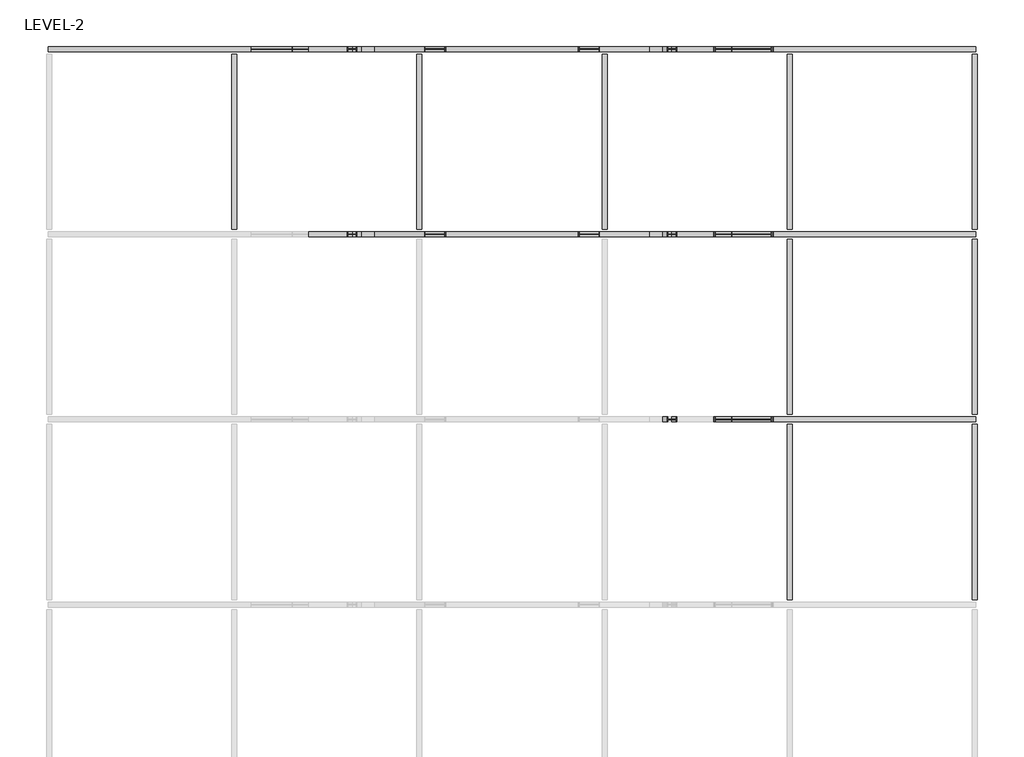
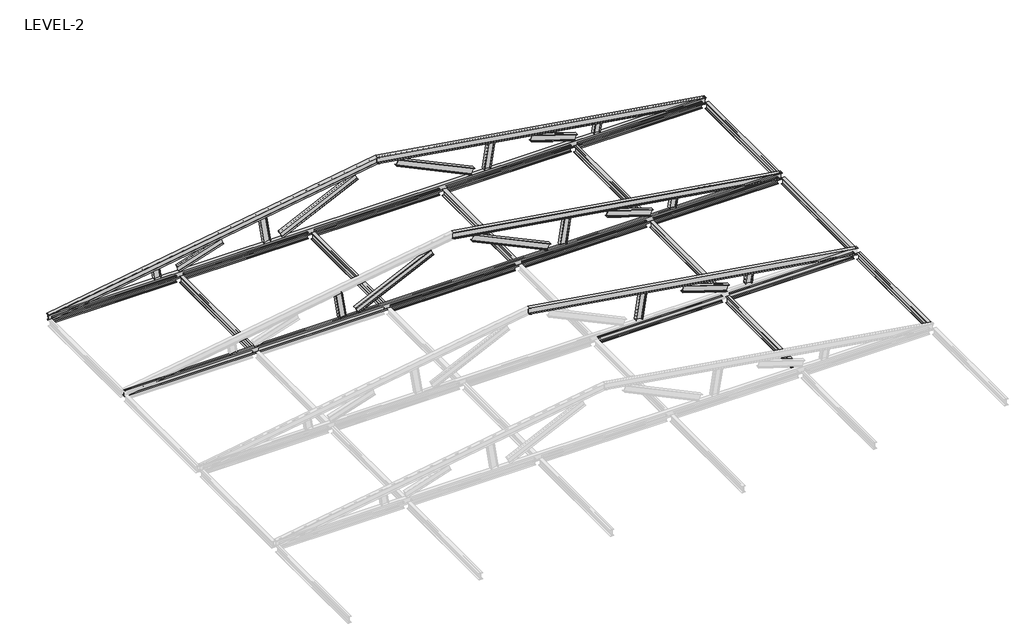
# One storey, part 3 of 3: 42 beams.
"""IFC4 building model written with IfcOpenShell, lengths in millimetres."""

from ifc_helpers import new_model, si_unit, frame, origin, place, context, project, spatial, polyline, circle_curve, ellipse_curve, transform, mapped, element, save
from ifc_brep_helpers import plane_surface, revolved_surface, advanced_brep
from components import ub_universal_beams_ub305x165x40_616d6e4e, ub_universal_beams_ub305x165x40_3f70edd5, ub_universal_beams_ub305x165x40_c9eec61f, ub_universal_beams_ub305x165x40_c956ba20, ub_universal_beams_ub305x165x40_f58164a9, ub_universal_beams_ub305x165x40_ef0a91e2, ub_universal_beams_ub305x165x40_83ed4f69, ub_universal_beams_ub305x165x40_46a3dc55, ub_universal_beams_ub305x165x40_0b6a72e4, ub_universal_beams_ub305x165x40_63d5ebb1, ub_universal_beams_ub305x165x40_05d28e63

model = new_model("IFC4")

# Units and contexts
model_context = context("Model", 3, world=origin())
ifc_project = project(units=[si_unit("LENGTHUNIT", "METRE", prefix="MILLI")], contexts=[model_context])

# Site, building, storey
site = spatial("IfcSite", under=ifc_project)
building = spatial("IfcBuilding", under=site)
storey = spatial("IfcBuildingStorey", under=building, Name="LEVEL-2", Elevation=4267.0)

# Beams
placement = place(None, origin())
element("IfcBeam", 1, ObjectType="UB-Universal Beams : UB305x165x40", at=placement, inside=storey, context=model_context, shape_type="AdvancedBrep", body=[
    advanced_brep(
    [(11917.6451312, 4042.0234105, 4127.2241081), (11917.6451312, 3971.4234105, 4127.2241081), (11919.0296431, 3962.5234105, 4136.0157591), (11960.2849884, 3962.5234105, 4397.9872012), (11961.6695003, 3971.4234105, 4406.7788522), (11961.6695003, 4042.0234105, 4406.7788522), (11963.2562444, 4042.0234105, 4416.8546768), (11963.2562444, 3877.0234105, 4416.8546768), (11961.6695003, 3877.0234105, 4406.7788522), (11961.6695003, 3947.6234105, 4406.7788522), (11960.2849884, 3956.5234105, 4397.9872012), (11919.0296431, 3956.5234105, 4136.0157591), (11917.6451312, 3947.6234105, 4127.2241081), (11917.6451312, 3877.0234105, 4127.2241081), (11916.0583871, 3877.0234105, 4117.1482834), (11916.0583871, 4042.0234105, 4117.1482834), (-3300.3332854, 4042.0234105, 6523.7561422), (-3300.3332854, 3971.4234105, 6523.7561422), (-3300.3332854, 3962.5234105, 6532.7658266), (-3300.3332854, 3962.5234105, 6801.2341734), (-3300.3332854, 3971.4234105, 6810.2438578), (-3300.3332854, 4042.0234105, 6810.2438578), (-3300.3332854, 4042.0234105, 6820.5695634), (-3300.3332854, 3877.0234105, 6820.5695634), (-3300.3332854, 3877.0234105, 6810.2438578), (-3300.3332854, 3947.6234105, 6810.2438578), (-3300.3332854, 3956.5234105, 6801.2341734), (-3300.3332854, 3956.5234105, 6532.7658266), (-3300.3332854, 3947.6234105, 6523.7561422), (-3300.3332854, 3877.0234105, 6523.7561422), (-3300.3332854, 3877.0234105, 6513.4304366), (-3300.3332854, 4042.0234105, 6513.4304366)],
    [
        (0, 1),
        (1, 2, circle_curve(frame((11919.0296431, 3971.4234105, 4136.0157591), z_axis=(-0.9878259507117182, 0.0, 0.1555631418443652), x_axis=(0.0, -1.0, 0.0)), 8.9)),
        (2, 3),
        (3, 4, circle_curve(frame((11960.2849884, 3971.4234105, 4397.9872012), z_axis=(-0.9878259507117182, 0.0, 0.1555631418443652), x_axis=(0.0, -1.0, 0.0)), 8.9)),
        (4, 5),
        (5, 6),
        (6, 7),
        (7, 8),
        (8, 9),
        (9, 10, circle_curve(frame((11960.2849884, 3947.6234105, 4397.9872012), z_axis=(-0.9878259507117182, 0.0, 0.1555631418443652), x_axis=(0.0, -1.0, 0.0)), 8.9)),
        (10, 11),
        (11, 12, circle_curve(frame((11919.0296431, 3947.6234105, 4136.0157591), z_axis=(-0.9878259507117182, 0.0, 0.1555631418443652), x_axis=(0.0, -1.0, 0.0)), 8.9)),
        (12, 13),
        (13, 14),
        (14, 15),
        (15, 0),
        (0, 16),
        (16, 17),
        (17, 1),
        (17, 18, ellipse_curve(frame((-3300.3332854, 3971.4234105, 6532.7658266), z_axis=(-1.0, 0.0, 0.0), x_axis=(0.0, 0.0, 1.0)), 9.0096843, 8.9)),
        (18, 2),
        (18, 19),
        (19, 3),
        (19, 20, ellipse_curve(frame((-3300.3332854, 3971.4234105, 6801.2341734), z_axis=(-1.0, 0.0, 0.0), x_axis=(0.0, 0.0, 1.0)), 9.0096843, 8.9)),
        (20, 4),
        (20, 21),
        (21, 5),
        (21, 22),
        (22, 6),
        (22, 23),
        (23, 7),
        (23, 24),
        (24, 8),
        (24, 25),
        (25, 9),
        (25, 26, ellipse_curve(frame((-3300.3332854, 3947.6234105, 6801.2341734), z_axis=(-1.0, 0.0, 0.0), x_axis=(0.0, 0.0, 1.0)), 9.0096843, 8.9)),
        (26, 10),
        (26, 27),
        (27, 11),
        (27, 28, ellipse_curve(frame((-3300.3332854, 3947.6234105, 6532.7658266), z_axis=(-1.0, 0.0, 0.0), x_axis=(0.0, 0.0, 1.0)), 9.0096843, 8.9)),
        (28, 12),
        (28, 29),
        (29, 13),
        (29, 30),
        (30, 14),
        (30, 31),
        (31, 15),
        (31, 16),
    ],
    [
        plane_surface(frame((11939.6573157, 3959.5234105, 4267.0014801), z_axis=(0.9878259507117182, 0.0, -0.1555631418443652), x_axis=(0.1555631418443652, 0.0, 0.9878259507117182))),
        plane_surface(frame((11917.6451312, 4042.0234105, 4127.2241081), z_axis=(0.1555631418443652, 0.0, 0.9878259507117182), x_axis=(-0.9878259507117182, 0.0, 0.1555631418443652))),
        revolved_surface(polyline([(-3301.7177973591024, 3962.5234105, 6532.983859959702), (11919.029643166847, 3962.5234105, 4136.015759089472)]), (11919.0296431, 3971.4234105, 4136.0157591), (-0.9878259507117182, 0.0, 0.1555631418443652)),
        plane_surface(frame((11919.0296431, 3962.5234105, 4136.0157591), z_axis=(0.0, 1.0, 0.0), x_axis=(-0.9878259507117182, 0.0, 0.1555631418443652))),
        revolved_surface(polyline([(-3301.717797363457, 3962.5234105, 6801.452206832042), (11960.2849884, 3962.5234105, 4397.9872012)]), (11960.2849884, 3971.4234105, 4397.9872012), (-0.9878259507117182, 0.0, 0.1555631418443652)),
        plane_surface(frame((11961.6695003, 3971.4234105, 4406.7788522), z_axis=(-0.1555631418443652, 0.0, -0.9878259507117182), x_axis=(-0.9878259507117182, 0.0, 0.1555631418443652))),
        plane_surface(frame((11961.6695003, 4042.0234105, 4406.7788522), z_axis=(0.0, 1.0, 0.0), x_axis=(-0.9878259507117182, 0.0, 0.1555631418443652))),
        plane_surface(frame((11963.2562444, 4042.0234105, 4416.8546768), z_axis=(0.1555631418443652, 0.0, 0.9878259507117182), x_axis=(-0.9878259507117182, 0.0, 0.1555631418443652))),
        plane_surface(frame((11963.2562444, 3877.0234105, 4416.8546768), z_axis=(0.0, -1.0, 0.0), x_axis=(-0.9878259507117182, 0.0, 0.1555631418443652))),
        plane_surface(frame((11961.6695003, 3877.0234105, 4406.7788522), z_axis=(-0.1555631418443652, 0.0, -0.9878259507117182), x_axis=(-0.9878259507117182, 0.0, 0.1555631418443652))),
        revolved_surface(polyline([(-3301.717797363457, 3938.7234104999998, 6801.452206832042), (11960.2849884, 3938.7234104999998, 4397.9872012)]), (11960.2849884, 3947.6234105, 4397.9872012), (-0.9878259507117182, 0.0, 0.1555631418443652)),
        plane_surface(frame((11960.2849884, 3956.5234105, 4397.9872012), z_axis=(0.0, -1.0, 0.0), x_axis=(-0.9878259507117182, 0.0, 0.1555631418443652))),
        revolved_surface(polyline([(-3301.7177973591024, 3938.7234104999998, 6532.983859959702), (11919.029643166847, 3938.7234104999998, 4136.015759089472)]), (11919.0296431, 3947.6234105, 4136.0157591), (-0.9878259507117182, 0.0, 0.1555631418443652)),
        plane_surface(frame((11917.6451312, 3947.6234105, 4127.2241081), z_axis=(0.1555631418443652, 0.0, 0.9878259507117182), x_axis=(-0.9878259507117182, 0.0, 0.1555631418443652))),
        plane_surface(frame((11917.6451312, 3877.0234105, 4127.2241081), z_axis=(0.0, -1.0, 0.0), x_axis=(-0.9878259507117182, 0.0, 0.1555631418443652))),
        plane_surface(frame((11916.0583871, 3877.0234105, 4117.1482834), z_axis=(-0.1555631418443652, 0.0, -0.9878259507117182), x_axis=(-0.9878259507117182, 0.0, 0.1555631418443652))),
        plane_surface(frame((11916.0583871, 4042.0234105, 4117.1482834), z_axis=(0.0, 1.0, 0.0), x_axis=(-0.9878259507117182, 0.0, 0.1555631418443652))),
        plane_surface(frame((-3300.3332854, 3959.5234105, 6820.5695634), z_axis=(-1.0, 0.0, 0.0), x_axis=(0.0, 1.0, 0.0))),
    ],
    [
        (0, [[1, 2, 3, 4, 5, 6, 7, 8, 9, 10, 11, 12, 13, 14, 15, 16]]),
        (1, [[-1, 17, 18, 19]]),
        (2, [[-2, -19, 20, 21]]),
        (3, [[-3, -21, 22, 23]]),
        (4, [[-4, -23, 24, 25]]),
        (5, [[-5, -25, 26, 27]]),
        (6, [[-6, -27, 28, 29]]),
        (7, [[-7, -29, 30, 31]]),
        (8, [[-8, -31, 32, 33]]),
        (9, [[-9, -33, 34, 35]]),
        (10, [[-10, -35, 36, 37]]),
        (11, [[-11, -37, 38, 39]]),
        (12, [[-12, -39, 40, 41]]),
        (13, [[-13, -41, 42, 43]]),
        (14, [[-14, -43, 44, 45]]),
        (15, [[-15, -45, 46, 47]]),
        (16, [[-16, -47, 48, -17]]),
        (17, [[-48, -46, -44, -42, -40, -38, -36, -34, -32, -30, -28, -26, -24, -22, -20, -18]]),
    ],
),
])
element("IfcBeam", 2, ObjectType="UB-Universal Beams : UB305x165x40", at=placement, inside=storey, context=model_context, shape_type="AdvancedBrep", body=[
    advanced_brep(
    [(11917.6451312, 10138.0234105, 4127.2241081), (11917.6451312, 10067.4234105, 4127.2241081), (11919.0296431, 10058.5234105, 4136.0157591), (11960.2849884, 10058.5234105, 4397.9872012), (11961.6695003, 10067.4234105, 4406.7788522), (11961.6695003, 10138.0234105, 4406.7788522), (11963.2562444, 10138.0234105, 4416.8546768), (11963.2562444, 9973.0234105, 4416.8546768), (11961.6695003, 9973.0234105, 4406.7788522), (11961.6695003, 10043.6234105, 4406.7788522), (11960.2849884, 10052.5234105, 4397.9872012), (11919.0296431, 10052.5234105, 4136.0157591), (11917.6451312, 10043.6234105, 4127.2241081), (11917.6451312, 9973.0234105, 4127.2241081), (11916.0583871, 9973.0234105, 4117.1482834), (11916.0583871, 10138.0234105, 4117.1482834), (-3300.3332854, 10138.0234105, 6523.7561422), (-3300.3332854, 10067.4234105, 6523.7561422), (-3300.3332854, 10058.5234105, 6532.7658266), (-3300.3332854, 10058.5234105, 6801.2341734), (-3300.3332854, 10067.4234105, 6810.2438578), (-3300.3332854, 10138.0234105, 6810.2438578), (-3300.3332854, 10138.0234105, 6820.5695634), (-3300.3332854, 9973.0234105, 6820.5695634), (-3300.3332854, 9973.0234105, 6810.2438578), (-3300.3332854, 10043.6234105, 6810.2438578), (-3300.3332854, 10052.5234105, 6801.2341734), (-3300.3332854, 10052.5234105, 6532.7658266), (-3300.3332854, 10043.6234105, 6523.7561422), (-3300.3332854, 9973.0234105, 6523.7561422), (-3300.3332854, 9973.0234105, 6513.4304366), (-3300.3332854, 10138.0234105, 6513.4304366)],
    [
        (0, 1),
        (1, 2, circle_curve(frame((11919.0296431, 10067.4234105, 4136.0157591), z_axis=(-0.9878259507117182, 0.0, 0.1555631418443652), x_axis=(0.0, -1.0, 0.0)), 8.9)),
        (2, 3),
        (3, 4, circle_curve(frame((11960.2849884, 10067.4234105, 4397.9872012), z_axis=(-0.9878259507117182, 0.0, 0.1555631418443652), x_axis=(0.0, -1.0, 0.0)), 8.9)),
        (4, 5),
        (5, 6),
        (6, 7),
        (7, 8),
        (8, 9),
        (9, 10, circle_curve(frame((11960.2849884, 10043.6234105, 4397.9872012), z_axis=(-0.9878259507117182, 0.0, 0.1555631418443652), x_axis=(0.0, -1.0, 0.0)), 8.9)),
        (10, 11),
        (11, 12, circle_curve(frame((11919.0296431, 10043.6234105, 4136.0157591), z_axis=(-0.9878259507117182, 0.0, 0.1555631418443652), x_axis=(0.0, -1.0, 0.0)), 8.9)),
        (12, 13),
        (13, 14),
        (14, 15),
        (15, 0),
        (0, 16),
        (16, 17),
        (17, 1),
        (17, 18, ellipse_curve(frame((-3300.3332854, 10067.4234105, 6532.7658266), z_axis=(-1.0, 0.0, 0.0), x_axis=(0.0, 0.0, 1.0)), 9.0096843, 8.9)),
        (18, 2),
        (18, 19),
        (19, 3),
        (19, 20, ellipse_curve(frame((-3300.3332854, 10067.4234105, 6801.2341734), z_axis=(-1.0, 0.0, 0.0), x_axis=(0.0, 0.0, 1.0)), 9.0096843, 8.9)),
        (20, 4),
        (20, 21),
        (21, 5),
        (21, 22),
        (22, 6),
        (22, 23),
        (23, 7),
        (23, 24),
        (24, 8),
        (24, 25),
        (25, 9),
        (25, 26, ellipse_curve(frame((-3300.3332854, 10043.6234105, 6801.2341734), z_axis=(-1.0, 0.0, 0.0), x_axis=(0.0, 0.0, 1.0)), 9.0096843, 8.9)),
        (26, 10),
        (26, 27),
        (27, 11),
        (27, 28, ellipse_curve(frame((-3300.3332854, 10043.6234105, 6532.7658266), z_axis=(-1.0, 0.0, 0.0), x_axis=(0.0, 0.0, 1.0)), 9.0096843, 8.9)),
        (28, 12),
        (28, 29),
        (29, 13),
        (29, 30),
        (30, 14),
        (30, 31),
        (31, 15),
        (31, 16),
    ],
    [
        plane_surface(frame((11939.6573157, 10055.5234105, 4267.0014801), z_axis=(0.9878259507117182, 0.0, -0.1555631418443652), x_axis=(0.1555631418443652, 0.0, 0.9878259507117182))),
        plane_surface(frame((11917.6451312, 10138.0234105, 4127.2241081), z_axis=(0.1555631418443652, 0.0, 0.9878259507117182), x_axis=(-0.9878259507117182, 0.0, 0.1555631418443652))),
        revolved_surface(polyline([(-3301.7177973591024, 10058.5234105, 6532.983859959702), (11919.029643166847, 10058.5234105, 4136.015759089472)]), (11919.0296431, 10067.4234105, 4136.0157591), (-0.9878259507117182, 0.0, 0.1555631418443652)),
        plane_surface(frame((11919.0296431, 10058.5234105, 4136.0157591), z_axis=(0.0, 1.0, 0.0), x_axis=(-0.9878259507117182, 0.0, 0.1555631418443652))),
        revolved_surface(polyline([(-3301.717797363457, 10058.5234105, 6801.452206832042), (11960.2849884, 10058.5234105, 4397.9872012)]), (11960.2849884, 10067.4234105, 4397.9872012), (-0.9878259507117182, 0.0, 0.1555631418443652)),
        plane_surface(frame((11961.6695003, 10067.4234105, 4406.7788522), z_axis=(-0.1555631418443652, 0.0, -0.9878259507117182), x_axis=(-0.9878259507117182, 0.0, 0.1555631418443652))),
        plane_surface(frame((11961.6695003, 10138.0234105, 4406.7788522), z_axis=(0.0, 1.0, 0.0), x_axis=(-0.9878259507117182, 0.0, 0.1555631418443652))),
        plane_surface(frame((11963.2562444, 10138.0234105, 4416.8546768), z_axis=(0.1555631418443652, 0.0, 0.9878259507117182), x_axis=(-0.9878259507117182, 0.0, 0.1555631418443652))),
        plane_surface(frame((11963.2562444, 9973.0234105, 4416.8546768), z_axis=(0.0, -1.0, 0.0), x_axis=(-0.9878259507117182, 0.0, 0.1555631418443652))),
        plane_surface(frame((11961.6695003, 9973.0234105, 4406.7788522), z_axis=(-0.1555631418443652, 0.0, -0.9878259507117182), x_axis=(-0.9878259507117182, 0.0, 0.1555631418443652))),
        revolved_surface(polyline([(-3301.717797363457, 10034.7234105, 6801.452206832042), (11960.2849884, 10034.7234105, 4397.9872012)]), (11960.2849884, 10043.6234105, 4397.9872012), (-0.9878259507117182, 0.0, 0.1555631418443652)),
        plane_surface(frame((11960.2849884, 10052.5234105, 4397.9872012), z_axis=(0.0, -1.0, 0.0), x_axis=(-0.9878259507117182, 0.0, 0.1555631418443652))),
        revolved_surface(polyline([(-3301.7177973591024, 10034.7234105, 6532.983859959702), (11919.029643166847, 10034.7234105, 4136.015759089472)]), (11919.0296431, 10043.6234105, 4136.0157591), (-0.9878259507117182, 0.0, 0.1555631418443652)),
        plane_surface(frame((11917.6451312, 10043.6234105, 4127.2241081), z_axis=(0.1555631418443652, 0.0, 0.9878259507117182), x_axis=(-0.9878259507117182, 0.0, 0.1555631418443652))),
        plane_surface(frame((11917.6451312, 9973.0234105, 4127.2241081), z_axis=(0.0, -1.0, 0.0), x_axis=(-0.9878259507117182, 0.0, 0.1555631418443652))),
        plane_surface(frame((11916.0583871, 9973.0234105, 4117.1482834), z_axis=(-0.1555631418443652, 0.0, -0.9878259507117182), x_axis=(-0.9878259507117182, 0.0, 0.1555631418443652))),
        plane_surface(frame((11916.0583871, 10138.0234105, 4117.1482834), z_axis=(0.0, 1.0, 0.0), x_axis=(-0.9878259507117182, 0.0, 0.1555631418443652))),
        plane_surface(frame((-3300.3332854, 10055.5234105, 6820.5695634), z_axis=(-1.0, 0.0, 0.0), x_axis=(0.0, 1.0, 0.0))),
    ],
    [
        (0, [[1, 2, 3, 4, 5, 6, 7, 8, 9, 10, 11, 12, 13, 14, 15, 16]]),
        (1, [[-1, 17, 18, 19]]),
        (2, [[-2, -19, 20, 21]]),
        (3, [[-3, -21, 22, 23]]),
        (4, [[-4, -23, 24, 25]]),
        (5, [[-5, -25, 26, 27]]),
        (6, [[-6, -27, 28, 29]]),
        (7, [[-7, -29, 30, 31]]),
        (8, [[-8, -31, 32, 33]]),
        (9, [[-9, -33, 34, 35]]),
        (10, [[-10, -35, 36, 37]]),
        (11, [[-11, -37, 38, 39]]),
        (12, [[-12, -39, 40, 41]]),
        (13, [[-13, -41, 42, 43]]),
        (14, [[-14, -43, 44, 45]]),
        (15, [[-15, -45, 46, 47]]),
        (16, [[-16, -47, 48, -17]]),
        (17, [[-48, -46, -44, -42, -40, -38, -36, -34, -32, -30, -28, -26, -24, -22, -20, -18]]),
    ],
),
])
element("IfcBeam", 3, ObjectType="UB-Universal Beams : UB305x165x40", at=placement, inside=storey, context=model_context, shape_type="AdvancedBrep", body=[
    advanced_brep(
    [(-18518.3117021, 16234.0234105, 4127.2241081), (-18516.724958, 16234.0234105, 4117.1482834), (-18516.724958, 16069.0234105, 4117.1482834), (-18518.3117021, 16069.0234105, 4127.2241081), (-18518.3117021, 16139.6234105, 4127.2241081), (-18519.696214, 16148.5234105, 4136.0157591), (-18560.9515593, 16148.5234105, 4397.9872012), (-18562.3360712, 16139.6234105, 4406.7788522), (-18562.3360712, 16069.0234105, 4406.7788522), (-18563.9228153, 16069.0234105, 4416.8546768), (-18563.9228153, 16234.0234105, 4416.8546768), (-18562.3360712, 16234.0234105, 4406.7788522), (-18562.3360712, 16163.4234105, 4406.7788522), (-18560.9515593, 16154.5234105, 4397.9872012), (-18519.696214, 16154.5234105, 4136.0157591), (-18518.3117021, 16163.4234105, 4127.2241081), (-3300.3332854, 16163.4234105, 6523.7561422), (-3300.3332854, 16234.0234105, 6523.7561422), (-3300.3332854, 16154.5234105, 6532.7658266), (-3300.3332854, 16154.5234105, 6801.2341734), (-3300.3332854, 16163.4234105, 6810.2438578), (-3300.3332854, 16234.0234105, 6810.2438578), (-3300.3332854, 16234.0234105, 6820.5695634), (-3300.3332854, 16069.0234105, 6820.5695634), (-3300.3332854, 16069.0234105, 6810.2438578), (-3300.3332854, 16139.6234105, 6810.2438578), (-3300.3332854, 16148.5234105, 6801.2341734), (-3300.3332854, 16148.5234105, 6532.7658266), (-3300.3332854, 16139.6234105, 6523.7561422), (-3300.3332854, 16069.0234105, 6523.7561422), (-3300.3332854, 16069.0234105, 6513.4304366), (-3300.3332854, 16234.0234105, 6513.4304366)],
    [
        (0, 1),
        (1, 2),
        (2, 3),
        (3, 4),
        (4, 5, circle_curve(frame((-18519.696214, 16139.6234105, 4136.0157591), z_axis=(0.9878259507117182, 0.0, 0.1555631418443652), x_axis=(0.0, -1.0, 0.0)), 8.9)),
        (5, 6),
        (6, 7, circle_curve(frame((-18560.9515593, 16139.6234105, 4397.9872012), z_axis=(0.9878259507117182, 0.0, 0.1555631418443652), x_axis=(0.0, -1.0, 0.0)), 8.9)),
        (7, 8),
        (8, 9),
        (9, 10),
        (10, 11),
        (11, 12),
        (12, 13, circle_curve(frame((-18560.9515593, 16163.4234105, 4397.9872012), z_axis=(0.9878259507117182, 0.0, 0.1555631418443652), x_axis=(0.0, -1.0, 0.0)), 8.9)),
        (13, 14),
        (14, 15, circle_curve(frame((-18519.696214, 16163.4234105, 4136.0157591), z_axis=(0.9878259507117182, 0.0, 0.1555631418443652), x_axis=(0.0, -1.0, 0.0)), 8.9)),
        (15, 0),
        (16, 17),
        (17, 0),
        (15, 16),
        (18, 16, ellipse_curve(frame((-3300.3332854, 16163.4234105, 6532.7658266), z_axis=(1.0, 0.0, 0.0), x_axis=(0.0, 0.0, -1.0)), 9.0096843, 8.9)),
        (14, 18),
        (19, 18),
        (13, 19),
        (20, 19, ellipse_curve(frame((-3300.3332854, 16163.4234105, 6801.2341734), z_axis=(1.0, 0.0, 0.0), x_axis=(0.0, 0.0, -1.0)), 9.0096843, 8.9)),
        (12, 20),
        (21, 20),
        (11, 21),
        (22, 21),
        (10, 22),
        (23, 22),
        (9, 23),
        (24, 23),
        (8, 24),
        (25, 24),
        (7, 25),
        (26, 25, ellipse_curve(frame((-3300.3332854, 16139.6234105, 6801.2341734), z_axis=(1.0, 0.0, 0.0), x_axis=(0.0, 0.0, -1.0)), 9.0096843, 8.9)),
        (6, 26),
        (27, 26),
        (5, 27),
        (28, 27, ellipse_curve(frame((-3300.3332854, 16139.6234105, 6532.7658266), z_axis=(1.0, 0.0, 0.0), x_axis=(0.0, 0.0, -1.0)), 9.0096843, 8.9)),
        (4, 28),
        (29, 28),
        (3, 29),
        (30, 29),
        (2, 30),
        (31, 30),
        (1, 31),
        (17, 31),
    ],
    [
        plane_surface(frame((-18540.3238866, 16151.5234105, 4267.0014801), z_axis=(-0.9878259507117182, 0.0, -0.1555631418443652), x_axis=(-0.1555631418443652, 0.0, 0.9878259507117182))),
        plane_surface(frame((-3278.3304997, 16234.0234105, 6527.2211478), z_axis=(-0.1555631418443652, 0.0, 0.9878259507117182), x_axis=(-0.9878259507117182, 0.0, -0.1555631418443652))),
        revolved_surface(polyline([(-18519.696214059466, 16154.5234105, 4136.015759042602), (-3298.948773435937, 16154.5234105, 6532.983859928199)]), (-3279.7150116, 16163.4234105, 6536.0127988), (-0.9878259507117182, 0.0, -0.1555631418443652)),
        plane_surface(frame((-3279.7150116, 16154.5234105, 6536.0127988), z_axis=(0.0, 1.0, 0.0), x_axis=(-0.9878259507117182, 0.0, -0.1555631418443652))),
        revolved_surface(polyline([(-18560.95155929262, 16154.5234105, 4397.98720115313), (-3298.948773431581, 16154.5234105, 6801.452206800539)]), (-3320.9703569, 16163.4234105, 6797.9842409), (-0.9878259507117182, 0.0, -0.1555631418443652)),
        plane_surface(frame((-3322.3548688, 16163.4234105, 6806.7758919), z_axis=(0.1555631418443652, 0.0, -0.9878259507117182), x_axis=(-0.9878259507117182, 0.0, -0.1555631418443652))),
        plane_surface(frame((-3322.3548688, 16234.0234105, 6806.7758919), z_axis=(0.0, 1.0, 0.0), x_axis=(-0.9878259507117182, 0.0, -0.1555631418443652))),
        plane_surface(frame((-3323.9416129, 16234.0234105, 6816.8517166), z_axis=(-0.1555631418443652, 0.0, 0.9878259507117182), x_axis=(-0.9878259507117182, 0.0, -0.1555631418443652))),
        plane_surface(frame((-3323.9416129, 16069.0234105, 6816.8517166), z_axis=(0.0, -1.0, 0.0), x_axis=(-0.9878259507117182, 0.0, -0.1555631418443652))),
        plane_surface(frame((-3322.3548688, 16069.0234105, 6806.7758919), z_axis=(0.1555631418443652, 0.0, -0.9878259507117182), x_axis=(-0.9878259507117182, 0.0, -0.1555631418443652))),
        revolved_surface(polyline([(-18560.95155929262, 16130.7234105, 4397.98720115313), (-3298.948773431581, 16130.7234105, 6801.452206800539)]), (-3320.9703569, 16139.6234105, 6797.9842409), (-0.9878259507117182, 0.0, -0.1555631418443652)),
        plane_surface(frame((-3320.9703569, 16148.5234105, 6797.9842409), z_axis=(0.0, -1.0, 0.0), x_axis=(-0.9878259507117182, 0.0, -0.1555631418443652))),
        revolved_surface(polyline([(-18519.696214059466, 16130.7234105, 4136.015759042602), (-3298.948773435937, 16130.7234105, 6532.983859928199)]), (-3279.7150116, 16139.6234105, 6536.0127988), (-0.9878259507117182, 0.0, -0.1555631418443652)),
        plane_surface(frame((-3278.3304997, 16139.6234105, 6527.2211478), z_axis=(-0.1555631418443652, 0.0, 0.9878259507117182), x_axis=(-0.9878259507117182, 0.0, -0.1555631418443652))),
        plane_surface(frame((-3278.3304997, 16069.0234105, 6527.2211478), z_axis=(0.0, -1.0, 0.0), x_axis=(-0.9878259507117182, 0.0, -0.1555631418443652))),
        plane_surface(frame((-3276.7437556, 16069.0234105, 6517.1453232), z_axis=(0.1555631418443652, 0.0, -0.9878259507117182), x_axis=(-0.9878259507117182, 0.0, -0.1555631418443652))),
        plane_surface(frame((-3276.7437556, 16234.0234105, 6517.1453232), z_axis=(0.0, 1.0, 0.0), x_axis=(-0.9878259507117182, 0.0, -0.1555631418443652))),
        plane_surface(frame((-3300.3332854, 16151.5234105, 6820.5695634), z_axis=(1.0, 0.0, 0.0), x_axis=(0.0, -1.0, 0.0))),
    ],
    [
        (0, [[1, 2, 3, 4, 5, 6, 7, 8, 9, 10, 11, 12, 13, 14, 15, 16]]),
        (1, [[17, 18, -16, 19]]),
        (2, [[20, -19, -15, 21]]),
        (3, [[22, -21, -14, 23]]),
        (4, [[24, -23, -13, 25]]),
        (5, [[26, -25, -12, 27]]),
        (6, [[28, -27, -11, 29]]),
        (7, [[30, -29, -10, 31]]),
        (8, [[32, -31, -9, 33]]),
        (9, [[34, -33, -8, 35]]),
        (10, [[36, -35, -7, 37]]),
        (11, [[38, -37, -6, 39]]),
        (12, [[40, -39, -5, 41]]),
        (13, [[42, -41, -4, 43]]),
        (14, [[44, -43, -3, 45]]),
        (15, [[46, -45, -2, 47]]),
        (16, [[48, -47, -1, -18]]),
        (17, [[-17, -20, -22, -24, -26, -28, -30, -32, -34, -36, -38, -40, -42, -44, -46, -48]]),
    ],
),
])
element("IfcBeam", 4, ObjectType="UB-Universal Beams : UB305x165x40", at=placement, inside=storey, context=model_context, shape_type="AdvancedBrep", body=[
    advanced_brep(
    [(11917.6451312, 16234.0234105, 4127.2241081), (11917.6451312, 16163.4234105, 4127.2241081), (11919.0296431, 16154.5234105, 4136.0157591), (11960.2849884, 16154.5234105, 4397.9872012), (11961.6695003, 16163.4234105, 4406.7788522), (11961.6695003, 16234.0234105, 4406.7788522), (11963.2562444, 16234.0234105, 4416.8546768), (11963.2562444, 16069.0234105, 4416.8546768), (11961.6695003, 16069.0234105, 4406.7788522), (11961.6695003, 16139.6234105, 4406.7788522), (11960.2849884, 16148.5234105, 4397.9872012), (11919.0296431, 16148.5234105, 4136.0157591), (11917.6451312, 16139.6234105, 4127.2241081), (11917.6451312, 16069.0234105, 4127.2241081), (11916.0583871, 16069.0234105, 4117.1482834), (11916.0583871, 16234.0234105, 4117.1482834), (-3300.3332854, 16234.0234105, 6523.7561422), (-3300.3332854, 16163.4234105, 6523.7561422), (-3300.3332854, 16154.5234105, 6532.7658266), (-3300.3332854, 16154.5234105, 6801.2341734), (-3300.3332854, 16163.4234105, 6810.2438578), (-3300.3332854, 16234.0234105, 6810.2438578), (-3300.3332854, 16234.0234105, 6820.5695634), (-3300.3332854, 16069.0234105, 6820.5695634), (-3300.3332854, 16069.0234105, 6810.2438578), (-3300.3332854, 16139.6234105, 6810.2438578), (-3300.3332854, 16148.5234105, 6801.2341734), (-3300.3332854, 16148.5234105, 6532.7658266), (-3300.3332854, 16139.6234105, 6523.7561422), (-3300.3332854, 16069.0234105, 6523.7561422), (-3300.3332854, 16069.0234105, 6513.4304366), (-3300.3332854, 16234.0234105, 6513.4304366)],
    [
        (0, 1),
        (1, 2, circle_curve(frame((11919.0296431, 16163.4234105, 4136.0157591), z_axis=(-0.9878259507117182, 0.0, 0.1555631418443652), x_axis=(0.0, -1.0, 0.0)), 8.9)),
        (2, 3),
        (3, 4, circle_curve(frame((11960.2849884, 16163.4234105, 4397.9872012), z_axis=(-0.9878259507117182, 0.0, 0.1555631418443652), x_axis=(0.0, -1.0, 0.0)), 8.9)),
        (4, 5),
        (5, 6),
        (6, 7),
        (7, 8),
        (8, 9),
        (9, 10, circle_curve(frame((11960.2849884, 16139.6234105, 4397.9872012), z_axis=(-0.9878259507117182, 0.0, 0.1555631418443652), x_axis=(0.0, -1.0, 0.0)), 8.9)),
        (10, 11),
        (11, 12, circle_curve(frame((11919.0296431, 16139.6234105, 4136.0157591), z_axis=(-0.9878259507117182, 0.0, 0.1555631418443652), x_axis=(0.0, -1.0, 0.0)), 8.9)),
        (12, 13),
        (13, 14),
        (14, 15),
        (15, 0),
        (0, 16),
        (16, 17),
        (17, 1),
        (17, 18, ellipse_curve(frame((-3300.3332854, 16163.4234105, 6532.7658266), z_axis=(-1.0, 0.0, 0.0), x_axis=(0.0, 0.0, 1.0)), 9.0096843, 8.9)),
        (18, 2),
        (18, 19),
        (19, 3),
        (19, 20, ellipse_curve(frame((-3300.3332854, 16163.4234105, 6801.2341734), z_axis=(-1.0, 0.0, 0.0), x_axis=(0.0, 0.0, 1.0)), 9.0096843, 8.9)),
        (20, 4),
        (20, 21),
        (21, 5),
        (21, 22),
        (22, 6),
        (22, 23),
        (23, 7),
        (23, 24),
        (24, 8),
        (24, 25),
        (25, 9),
        (25, 26, ellipse_curve(frame((-3300.3332854, 16139.6234105, 6801.2341734), z_axis=(-1.0, 0.0, 0.0), x_axis=(0.0, 0.0, 1.0)), 9.0096843, 8.9)),
        (26, 10),
        (26, 27),
        (27, 11),
        (27, 28, ellipse_curve(frame((-3300.3332854, 16139.6234105, 6532.7658266), z_axis=(-1.0, 0.0, 0.0), x_axis=(0.0, 0.0, 1.0)), 9.0096843, 8.9)),
        (28, 12),
        (28, 29),
        (29, 13),
        (29, 30),
        (30, 14),
        (30, 31),
        (31, 15),
        (31, 16),
    ],
    [
        plane_surface(frame((11939.6573157, 16151.5234105, 4267.0014801), z_axis=(0.9878259507117182, 0.0, -0.1555631418443652), x_axis=(0.1555631418443652, 0.0, 0.9878259507117182))),
        plane_surface(frame((11917.6451312, 16234.0234105, 4127.2241081), z_axis=(0.1555631418443652, 0.0, 0.9878259507117182), x_axis=(-0.9878259507117182, 0.0, 0.1555631418443652))),
        revolved_surface(polyline([(-3301.7177973591024, 16154.5234105, 6532.983859959702), (11919.029643166847, 16154.5234105, 4136.015759089472)]), (11919.0296431, 16163.4234105, 4136.0157591), (-0.9878259507117182, 0.0, 0.1555631418443652)),
        plane_surface(frame((11919.0296431, 16154.5234105, 4136.0157591), z_axis=(0.0, 1.0, 0.0), x_axis=(-0.9878259507117182, 0.0, 0.1555631418443652))),
        revolved_surface(polyline([(-3301.717797363457, 16154.5234105, 6801.452206832042), (11960.2849884, 16154.5234105, 4397.9872012)]), (11960.2849884, 16163.4234105, 4397.9872012), (-0.9878259507117182, 0.0, 0.1555631418443652)),
        plane_surface(frame((11961.6695003, 16163.4234105, 4406.7788522), z_axis=(-0.1555631418443652, 0.0, -0.9878259507117182), x_axis=(-0.9878259507117182, 0.0, 0.1555631418443652))),
        plane_surface(frame((11961.6695003, 16234.0234105, 4406.7788522), z_axis=(0.0, 1.0, 0.0), x_axis=(-0.9878259507117182, 0.0, 0.1555631418443652))),
        plane_surface(frame((11963.2562444, 16234.0234105, 4416.8546768), z_axis=(0.1555631418443652, 0.0, 0.9878259507117182), x_axis=(-0.9878259507117182, 0.0, 0.1555631418443652))),
        plane_surface(frame((11963.2562444, 16069.0234105, 4416.8546768), z_axis=(0.0, -1.0, 0.0), x_axis=(-0.9878259507117182, 0.0, 0.1555631418443652))),
        plane_surface(frame((11961.6695003, 16069.0234105, 4406.7788522), z_axis=(-0.1555631418443652, 0.0, -0.9878259507117182), x_axis=(-0.9878259507117182, 0.0, 0.1555631418443652))),
        revolved_surface(polyline([(-3301.717797363457, 16130.7234105, 6801.452206832042), (11960.2849884, 16130.7234105, 4397.9872012)]), (11960.2849884, 16139.6234105, 4397.9872012), (-0.9878259507117182, 0.0, 0.1555631418443652)),
        plane_surface(frame((11960.2849884, 16148.5234105, 4397.9872012), z_axis=(0.0, -1.0, 0.0), x_axis=(-0.9878259507117182, 0.0, 0.1555631418443652))),
        revolved_surface(polyline([(-3301.7177973591024, 16130.7234105, 6532.983859959702), (11919.029643166847, 16130.7234105, 4136.015759089472)]), (11919.0296431, 16139.6234105, 4136.0157591), (-0.9878259507117182, 0.0, 0.1555631418443652)),
        plane_surface(frame((11917.6451312, 16139.6234105, 4127.2241081), z_axis=(0.1555631418443652, 0.0, 0.9878259507117182), x_axis=(-0.9878259507117182, 0.0, 0.1555631418443652))),
        plane_surface(frame((11917.6451312, 16069.0234105, 4127.2241081), z_axis=(0.0, -1.0, 0.0), x_axis=(-0.9878259507117182, 0.0, 0.1555631418443652))),
        plane_surface(frame((11916.0583871, 16069.0234105, 4117.1482834), z_axis=(-0.1555631418443652, 0.0, -0.9878259507117182), x_axis=(-0.9878259507117182, 0.0, 0.1555631418443652))),
        plane_surface(frame((11916.0583871, 16234.0234105, 4117.1482834), z_axis=(0.0, 1.0, 0.0), x_axis=(-0.9878259507117182, 0.0, 0.1555631418443652))),
        plane_surface(frame((-3300.3332854, 16151.5234105, 6820.5695634), z_axis=(-1.0, 0.0, 0.0), x_axis=(0.0, 1.0, 0.0))),
    ],
    [
        (0, [[1, 2, 3, 4, 5, 6, 7, 8, 9, 10, 11, 12, 13, 14, 15, 16]]),
        (1, [[-1, 17, 18, 19]]),
        (2, [[-2, -19, 20, 21]]),
        (3, [[-3, -21, 22, 23]]),
        (4, [[-4, -23, 24, 25]]),
        (5, [[-5, -25, 26, 27]]),
        (6, [[-6, -27, 28, 29]]),
        (7, [[-7, -29, 30, 31]]),
        (8, [[-8, -31, 32, 33]]),
        (9, [[-9, -33, 34, 35]]),
        (10, [[-10, -35, 36, 37]]),
        (11, [[-11, -37, 38, 39]]),
        (12, [[-12, -39, 40, 41]]),
        (13, [[-13, -41, 42, 43]]),
        (14, [[-14, -43, 44, 45]]),
        (15, [[-15, -45, 46, 47]]),
        (16, [[-16, -47, 48, -17]]),
        (17, [[-48, -46, -44, -42, -40, -38, -36, -34, -32, -30, -28, -26, -24, -22, -20, -18]]),
    ],
),
])
ub_universal_beams_ub305x165x40_shape = ub_universal_beams_ub305x165x40_616d6e4e(model_context)
element("IfcBeam", 5, ObjectType="UB-Universal Beams : UB305x165x40", at=placement, inside=storey, context=model_context, shape_type="MappedRepresentation", body=[
    mapped(ub_universal_beams_ub305x165x40_shape, transform((2795.6667146, 3959.5234105, 4115.3), x_axis=(1.0, 0.0, 0.0), y_axis=(0.0, 1.0, 0.0), z_axis=(0.0, 0.0, 1.0))),
])
element("IfcBeam", 6, ObjectType="UB-Universal Beams : UB305x165x40", at=placement, inside=storey, context=model_context, shape_type="MappedRepresentation", body=[
    mapped(ub_universal_beams_ub305x165x40_shape, transform((8891.6667146, 3959.5234105, 4115.3), x_axis=(1.0, 0.0, 0.0), y_axis=(0.0, 1.0, 0.0), z_axis=(0.0, 0.0, 1.0))),
])
element("IfcBeam", 7, ObjectType="UB-Universal Beams : UB305x165x40", at=placement, inside=storey, context=model_context, shape_type="MappedRepresentation", body=[
    mapped(ub_universal_beams_ub305x165x40_shape, transform((-3300.3332854, 10055.5234105, 4115.3), x_axis=(1.0, 0.0, 0.0), y_axis=(0.0, 1.0, 0.0), z_axis=(0.0, 0.0, 1.0))),
])
element("IfcBeam", 8, ObjectType="UB-Universal Beams : UB305x165x40", at=placement, inside=storey, context=model_context, shape_type="MappedRepresentation", body=[
    mapped(ub_universal_beams_ub305x165x40_shape, transform((2795.6667146, 10055.5234105, 4115.3), x_axis=(1.0, 0.0, 0.0), y_axis=(0.0, 1.0, 0.0), z_axis=(0.0, 0.0, 1.0))),
])
element("IfcBeam", 9, ObjectType="UB-Universal Beams : UB305x165x40", at=placement, inside=storey, context=model_context, shape_type="MappedRepresentation", body=[
    mapped(ub_universal_beams_ub305x165x40_shape, transform((8891.6667146, 10055.5234105, 4115.3), x_axis=(1.0, 0.0, 0.0), y_axis=(0.0, 1.0, 0.0), z_axis=(0.0, 0.0, 1.0))),
])
element("IfcBeam", 10, ObjectType="UB-Universal Beams : UB305x165x40", at=placement, inside=storey, context=model_context, shape_type="MappedRepresentation", body=[
    mapped(ub_universal_beams_ub305x165x40_shape, transform((-15492.3332854, 16151.5234105, 4115.3), x_axis=(1.0, 0.0, 0.0), y_axis=(0.0, 1.0, 0.0), z_axis=(0.0, 0.0, 1.0))),
])
element("IfcBeam", 11, ObjectType="UB-Universal Beams : UB305x165x40", at=placement, inside=storey, context=model_context, shape_type="MappedRepresentation", body=[
    mapped(ub_universal_beams_ub305x165x40_shape, transform((-9396.3332854, 16151.5234105, 4115.3), x_axis=(1.0, 0.0, 0.0), y_axis=(0.0, 1.0, 0.0), z_axis=(0.0, 0.0, 1.0))),
])
element("IfcBeam", 12, ObjectType="UB-Universal Beams : UB305x165x40", at=placement, inside=storey, context=model_context, shape_type="MappedRepresentation", body=[
    mapped(ub_universal_beams_ub305x165x40_shape, transform((-3300.3332854, 16151.5234105, 4115.3), x_axis=(1.0, 0.0, 0.0), y_axis=(0.0, 1.0, 0.0), z_axis=(0.0, 0.0, 1.0))),
])
element("IfcBeam", 13, ObjectType="UB-Universal Beams : UB305x165x40", at=placement, inside=storey, context=model_context, shape_type="MappedRepresentation", body=[
    mapped(ub_universal_beams_ub305x165x40_shape, transform((2795.6667146, 16151.5234105, 4115.3), x_axis=(1.0, 0.0, 0.0), y_axis=(0.0, 1.0, 0.0), z_axis=(0.0, 0.0, 1.0))),
])
element("IfcBeam", 14, ObjectType="UB-Universal Beams : UB305x165x40", at=placement, inside=storey, context=model_context, shape_type="MappedRepresentation", body=[
    mapped(ub_universal_beams_ub305x165x40_shape, transform((8891.6667146, 16151.5234105, 4115.3), x_axis=(1.0, 0.0, 0.0), y_axis=(0.0, 1.0, 0.0), z_axis=(0.0, 0.0, 1.0))),
])
ub_universal_beams_ub305x165x40_2_shape = ub_universal_beams_ub305x165x40_3f70edd5(model_context)
element("IfcBeam", 15, ObjectType="UB-Universal Beams : UB305x165x40", at=placement, inside=storey, context=model_context, shape_type="MappedRepresentation", body=[
    mapped(ub_universal_beams_ub305x165x40_2_shape, transform((11939.6667146, 911.5234105, 4115.3), x_axis=(0.0, 1.0, 0.0), y_axis=(-1.0, 0.0, 0.0), z_axis=(0.0, 0.0, 1.0))),
])
element("IfcBeam", 16, ObjectType="UB-Universal Beams : UB305x165x40", at=placement, inside=storey, context=model_context, shape_type="MappedRepresentation", body=[
    mapped(ub_universal_beams_ub305x165x40_2_shape, transform((11939.6667146, 7007.5234105, 4115.3), x_axis=(0.0, 1.0, 0.0), y_axis=(-1.0, 0.0, 0.0), z_axis=(0.0, 0.0, 1.0))),
])
element("IfcBeam", 17, ObjectType="UB-Universal Beams : UB305x165x40", at=placement, inside=storey, context=model_context, shape_type="MappedRepresentation", body=[
    mapped(ub_universal_beams_ub305x165x40_2_shape, transform((11939.6667146, 13103.5234105, 4115.3), x_axis=(0.0, 1.0, 0.0), y_axis=(-1.0, 0.0, 0.0), z_axis=(0.0, 0.0, 1.0))),
])
element("IfcBeam", 18, ObjectType="UB-Universal Beams : UB305x165x40", at=placement, inside=storey, context=model_context, shape_type="MappedRepresentation", body=[
    mapped(ub_universal_beams_ub305x165x40_2_shape, transform((5843.6667146, 911.5234105, 4115.3), x_axis=(0.0, 1.0, 0.0), y_axis=(-1.0, 0.0, 0.0), z_axis=(0.0, 0.0, 1.0))),
])
element("IfcBeam", 19, ObjectType="UB-Universal Beams : UB305x165x40", at=placement, inside=storey, context=model_context, shape_type="MappedRepresentation", body=[
    mapped(ub_universal_beams_ub305x165x40_2_shape, transform((5843.6667146, 7007.5234105, 4115.3), x_axis=(0.0, 1.0, 0.0), y_axis=(-1.0, 0.0, 0.0), z_axis=(0.0, 0.0, 1.0))),
])
element("IfcBeam", 20, ObjectType="UB-Universal Beams : UB305x165x40", at=placement, inside=storey, context=model_context, shape_type="MappedRepresentation", body=[
    mapped(ub_universal_beams_ub305x165x40_2_shape, transform((5843.6667146, 13103.5234105, 4115.3), x_axis=(0.0, 1.0, 0.0), y_axis=(-1.0, 0.0, 0.0), z_axis=(0.0, 0.0, 1.0))),
])
element("IfcBeam", 21, ObjectType="UB-Universal Beams : UB305x165x40", at=placement, inside=storey, context=model_context, shape_type="MappedRepresentation", body=[
    mapped(ub_universal_beams_ub305x165x40_2_shape, transform((-252.3332854, 13103.5234105, 4115.3), x_axis=(0.0, 1.0, 0.0), y_axis=(-1.0, 0.0, 0.0), z_axis=(0.0, 0.0, 1.0))),
])
element("IfcBeam", 22, ObjectType="UB-Universal Beams : UB305x165x40", at=placement, inside=storey, context=model_context, shape_type="MappedRepresentation", body=[
    mapped(ub_universal_beams_ub305x165x40_2_shape, transform((-6348.3332854, 13103.5234105, 4115.3), x_axis=(0.0, 1.0, 0.0), y_axis=(-1.0, 0.0, 0.0), z_axis=(0.0, 0.0, 1.0))),
])
element("IfcBeam", 23, ObjectType="UB-Universal Beams : UB305x165x40", at=placement, inside=storey, context=model_context, shape_type="MappedRepresentation", body=[
    mapped(ub_universal_beams_ub305x165x40_2_shape, transform((-12444.3332854, 13103.5234105, 4115.3), x_axis=(0.0, 1.0, 0.0), y_axis=(-1.0, 0.0, 0.0), z_axis=(0.0, 0.0, 1.0))),
])
ub_universal_beams_ub305x165x40_3_shape = ub_universal_beams_ub305x165x40_c9eec61f(model_context)
element("IfcBeam", 24, ObjectType="UB-Universal Beams : UB305x165x40", at=placement, inside=storey, context=model_context, shape_type="MappedRepresentation", body=[
    mapped(ub_universal_beams_ub305x165x40_3_shape, transform((-3300.3332854, 10055.5234105, 4267.0), x_axis=(1.0, 0.0, 0.0), y_axis=(0.0, 1.0, 0.0), z_axis=(0.0, 0.0, 1.0))),
])
element("IfcBeam", 25, ObjectType="UB-Universal Beams : UB305x165x40", at=placement, inside=storey, context=model_context, shape_type="MappedRepresentation", body=[
    mapped(ub_universal_beams_ub305x165x40_3_shape, transform((-3300.3332854, 16151.5234105, 4267.0), x_axis=(1.0, 0.0, 0.0), y_axis=(0.0, 1.0, 0.0), z_axis=(0.0, 0.0, 1.0))),
])
ub_universal_beams_ub305x165x40_4_shape = ub_universal_beams_ub305x165x40_c956ba20(model_context)
element("IfcBeam", 26, ObjectType="UB-Universal Beams : UB305x165x40", at=placement, inside=storey, context=model_context, shape_type="MappedRepresentation", body=[
    mapped(ub_universal_beams_ub305x165x40_4_shape, transform((-5840.3332854, 10055.5234105, 5467.0), x_axis=(0.9041722720767189, 0.0, 0.427168002555931), y_axis=(0.0, -1.0, 0.0), z_axis=(0.427168002555931, 0.0, -0.9041722720767189))),
])
element("IfcBeam", 27, ObjectType="UB-Universal Beams : UB305x165x40", at=placement, inside=storey, context=model_context, shape_type="MappedRepresentation", body=[
    mapped(ub_universal_beams_ub305x165x40_4_shape, transform((-5840.3332854, 16151.5234105, 5467.0), x_axis=(0.9041722720767189, 0.0, 0.427168002555931), y_axis=(0.0, -1.0, 0.0), z_axis=(0.427168002555931, 0.0, -0.9041722720767189))),
])
ub_universal_beams_ub305x165x40_5_shape = ub_universal_beams_ub305x165x40_f58164a9(model_context)
element("IfcBeam", 28, ObjectType="UB-Universal Beams : UB305x165x40", at=placement, inside=storey, context=model_context, shape_type="MappedRepresentation", body=[
    mapped(ub_universal_beams_ub305x165x40_5_shape, transform((-760.3332854, 10055.5234105, 5467.0), x_axis=(0.9041722720767189, 0.0, -0.427168002555931), y_axis=(0.0, -1.0, 0.0), z_axis=(-0.427168002555931, 0.0, -0.9041722720767189))),
])
element("IfcBeam", 29, ObjectType="UB-Universal Beams : UB305x165x40", at=placement, inside=storey, context=model_context, shape_type="MappedRepresentation", body=[
    mapped(ub_universal_beams_ub305x165x40_5_shape, transform((-760.3332854, 16151.5234105, 5467.0), x_axis=(0.9041722720767189, 0.0, -0.427168002555931), y_axis=(0.0, -1.0, 0.0), z_axis=(-0.427168002555931, 0.0, -0.9041722720767189))),
])
ub_universal_beams_ub305x165x40_6_shape = ub_universal_beams_ub305x165x40_ef0a91e2(model_context)
element("IfcBeam", 30, ObjectType="UB-Universal Beams : UB305x165x40", at=placement, inside=storey, context=model_context, shape_type="MappedRepresentation", body=[
    mapped(ub_universal_beams_ub305x165x40_6_shape, transform((-8503.2687322, 10055.5234105, 5047.6400871), x_axis=(0.15556314184436565, 0.0, -0.9878259507117181), y_axis=(0.0, -1.0, 0.0), z_axis=(-0.9878259507117181, 0.0, -0.15556314184436565))),
])
element("IfcBeam", 31, ObjectType="UB-Universal Beams : UB305x165x40", at=placement, inside=storey, context=model_context, shape_type="MappedRepresentation", body=[
    mapped(ub_universal_beams_ub305x165x40_6_shape, transform((-8503.2687322, 16151.5234105, 5047.6400871), x_axis=(0.15556314184436565, 0.0, -0.9878259507117181), y_axis=(0.0, -1.0, 0.0), z_axis=(-0.9878259507117181, 0.0, -0.15556314184436565))),
])
ub_universal_beams_ub305x165x40_7_shape = ub_universal_beams_ub305x165x40_83ed4f69(model_context)
element("IfcBeam", 32, ObjectType="UB-Universal Beams : UB305x165x40", at=placement, inside=storey, context=model_context, shape_type="MappedRepresentation", body=[
    mapped(ub_universal_beams_ub305x165x40_7_shape, transform((1902.6021613, 3959.5234105, 5047.6400871), x_axis=(0.15556314184436432, 0.0, 0.9878259507117182), y_axis=(0.0, -1.0, 0.0), z_axis=(0.9878259507117182, 0.0, -0.15556314184436432))),
])
element("IfcBeam", 33, ObjectType="UB-Universal Beams : UB305x165x40", at=placement, inside=storey, context=model_context, shape_type="MappedRepresentation", body=[
    mapped(ub_universal_beams_ub305x165x40_7_shape, transform((1902.6021613, 10055.5234105, 5047.6400871), x_axis=(0.15556314184436432, 0.0, 0.9878259507117182), y_axis=(0.0, -1.0, 0.0), z_axis=(0.9878259507117182, 0.0, -0.15556314184436432))),
])
element("IfcBeam", 34, ObjectType="UB-Universal Beams : UB305x165x40", at=placement, inside=storey, context=model_context, shape_type="MappedRepresentation", body=[
    mapped(ub_universal_beams_ub305x165x40_7_shape, transform((1902.6021613, 16151.5234105, 5047.6400871), x_axis=(0.15556314184436432, 0.0, 0.9878259507117182), y_axis=(0.0, -1.0, 0.0), z_axis=(0.9878259507117182, 0.0, -0.15556314184436432))),
])
ub_universal_beams_ub305x165x40_8_shape = ub_universal_beams_ub305x165x40_46a3dc55(model_context)
element("IfcBeam", 35, ObjectType="UB-Universal Beams : UB305x165x40", at=placement, inside=storey, context=model_context, shape_type="MappedRepresentation", body=[
    mapped(ub_universal_beams_ub305x165x40_8_shape, transform((-11043.2687322, 16151.5234105, 5047.6400871), x_axis=(0.9516002177990198, 0.0, 0.307338616976224), y_axis=(0.0, -1.0, 0.0), z_axis=(0.307338616976224, 0.0, -0.9516002177990198))),
])
ub_universal_beams_ub305x165x40_9_shape = ub_universal_beams_ub305x165x40_0b6a72e4(model_context)
element("IfcBeam", 36, ObjectType="UB-Universal Beams : UB305x165x40", at=placement, inside=storey, context=model_context, shape_type="MappedRepresentation", body=[
    mapped(ub_universal_beams_ub305x165x40_9_shape, transform((4442.6021613, 3959.5234105, 5047.6400871), x_axis=(0.9516002177990198, 0.0, -0.307338616976224), y_axis=(0.0, -1.0, 0.0), z_axis=(-0.307338616976224, 0.0, -0.9516002177990198))),
])
element("IfcBeam", 37, ObjectType="UB-Universal Beams : UB305x165x40", at=placement, inside=storey, context=model_context, shape_type="MappedRepresentation", body=[
    mapped(ub_universal_beams_ub305x165x40_9_shape, transform((4442.6021613, 10055.5234105, 5047.6400871), x_axis=(0.9516002177990198, 0.0, -0.307338616976224), y_axis=(0.0, -1.0, 0.0), z_axis=(-0.307338616976224, 0.0, -0.9516002177990198))),
])
element("IfcBeam", 38, ObjectType="UB-Universal Beams : UB305x165x40", at=placement, inside=storey, context=model_context, shape_type="MappedRepresentation", body=[
    mapped(ub_universal_beams_ub305x165x40_9_shape, transform((4442.6021613, 16151.5234105, 5047.6400871), x_axis=(0.9516002177990198, 0.0, -0.307338616976224), y_axis=(0.0, -1.0, 0.0), z_axis=(-0.307338616976224, 0.0, -0.9516002177990198))),
])
ub_universal_beams_ub305x165x40_10_shape = ub_universal_beams_ub305x165x40_63d5ebb1(model_context)
element("IfcBeam", 39, ObjectType="UB-Universal Beams : UB305x165x40", at=placement, inside=storey, context=model_context, shape_type="MappedRepresentation", body=[
    mapped(ub_universal_beams_ub305x165x40_10_shape, transform((6921.1344379, 3959.5234105, 4657.3200436), x_axis=(0.1555631418443628, 0.0, 0.9878259507117186), y_axis=(0.0, -1.0, 0.0), z_axis=(0.9878259507117186, 0.0, -0.1555631418443628))),
])
element("IfcBeam", 40, ObjectType="UB-Universal Beams : UB305x165x40", at=placement, inside=storey, context=model_context, shape_type="MappedRepresentation", body=[
    mapped(ub_universal_beams_ub305x165x40_10_shape, transform((6921.1344379, 10055.5234105, 4657.3200436), x_axis=(0.1555631418443628, 0.0, 0.9878259507117186), y_axis=(0.0, -1.0, 0.0), z_axis=(0.9878259507117186, 0.0, -0.1555631418443628))),
])
element("IfcBeam", 41, ObjectType="UB-Universal Beams : UB305x165x40", at=placement, inside=storey, context=model_context, shape_type="MappedRepresentation", body=[
    mapped(ub_universal_beams_ub305x165x40_10_shape, transform((6921.1344379, 16151.5234105, 4657.3200436), x_axis=(0.1555631418443628, 0.0, 0.9878259507117186), y_axis=(0.0, -1.0, 0.0), z_axis=(0.9878259507117186, 0.0, -0.1555631418443628))),
])
ub_universal_beams_ub305x165x40_11_shape = ub_universal_beams_ub305x165x40_05d28e63(model_context)
element("IfcBeam", 42, ObjectType="UB-Universal Beams : UB305x165x40", at=placement, inside=storey, context=model_context, shape_type="MappedRepresentation", body=[
    mapped(ub_universal_beams_ub305x165x40_11_shape, transform((-13521.8010088, 16151.5234105, 4657.3200436), x_axis=(0.15556314184436565, 0.0, -0.9878259507117181), y_axis=(0.0, -1.0, 0.0), z_axis=(-0.9878259507117181, 0.0, -0.15556314184436565))),
])

save(model, "model.ifc")

# Revit data of these elements
# Type "UB-Universal Beams : UB305x165x40"
#   Section Name Key = "UB305X165X40"
#   Width = 16.5 cm
#   Web Thickness = 0.6 cm
#   Web Fillet = 0.89 cm
#   Warping Constant = 164000.0 cm⁶
#   Torsional Moment of Inertia = 14.70 cm⁴
#   Section Area = 51.3 cm²
#   Plastic Modulus weak axis = 142.0 cm³
#   Plastic Modulus strong axis = 623.0 cm³
#   Nominal Weight = 40.2999 kgf/m
#   Moment of Inertia weak axis = 764.00 cm⁴
#   Moment of Inertia strong axis = 8503.00 cm⁴
#   Height = 30.34 cm
#   Flange Thickness = 1.02 cm
#   Elastic Modulus weak axis = 92.6 cm³
#   Elastic Modulus strong axis = 560.0 cm³
#   Centroid Vertical = 15.17 cm
#   Centroid Horizontal = 8.25 cm
#   Bolt Spacing = 9.0 cm
#   Length [instance default] = 1500 mm
#   Structural Material [instance default] = Metal - Steel 43-275
#   Type Comments = ""
#   Assembly Code = ""
# Elements 1, 2, 3, 4, 5, 6, 7, 8, 9, 10, 11, 12, 13, 14, 15, 16, 17, 18, 19, 20, 21, 22, 23, 24, 25, 26, 27, 28, 29, 30, 31, 32, 33, 34, 35, 36, 37, 38, 39, 40, 41, 42 (IfcBeam, "UB-Universal Beams : UB305x165x40")
#   Structural Material = Metal - Steel 43-275
#   Phase Created = New Construction
#   Materials on its faces: "Metal - Steel 43-275"
# Materials
#   "Metal - Steel 43-275": class "Metal", colour RGB 247 247 247, transparency 0, Cost = 0
